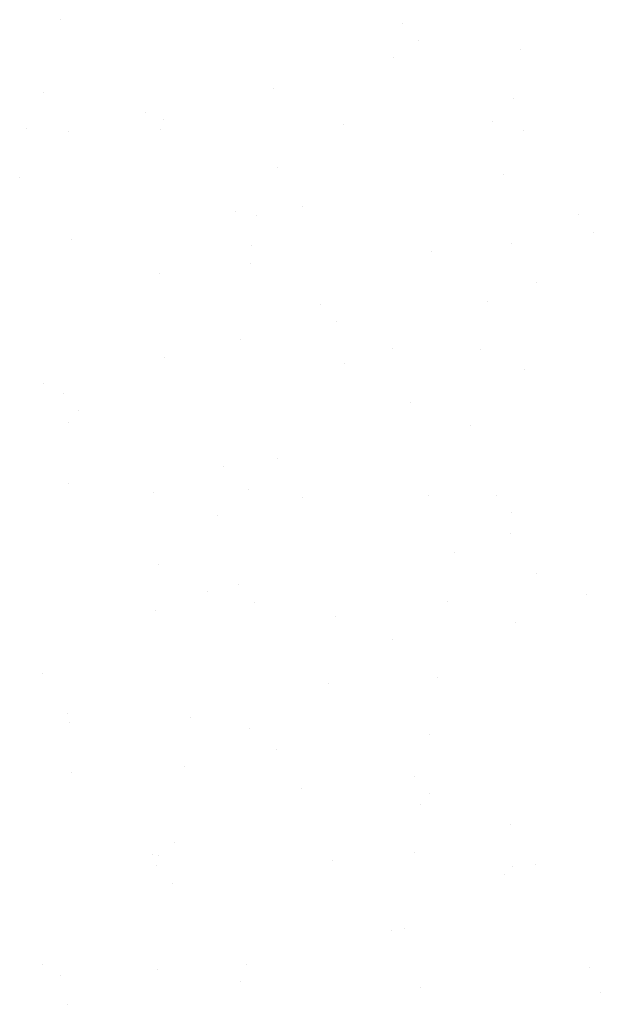
# Model space of a CAD drawing. Units: millimetres. Extents: x -857 to 54106, y -13666 to 13947.
# Tile 31 of 41: x 31340 to 31621, y 8976 to 9452. Entities that reach past the tile are written whole.
import ezdxf

# ---------------------------------------------------------------- set-up
doc = ezdxf.new("R2010")
doc.units = ezdxf.units.MM
doc.layers.add('A-FURN', color=21, linetype='Continuous', lineweight=18)
doc.layers.add('A-HT', color=15, linetype='Continuous')

# ---------------------------------------------------------------- blocks, each defined once
blk = doc.blocks.new('*X18')
at = {"color": 0}
for p, q in [((2.42041, 2.51943), (2.42041, 2.51943)), ((2.44643, 2.52286), (2.44643, 2.52286)), ((2.40072, 2.51004), (2.40072, 2.51004)), ((2.55643, 2.51033), (2.55643, 2.51033)), ((2.71213, 2.51061), (2.71213, 2.51061)), ((2.86784, 2.51089), (2.86784, 2.51089)), ((2.36196, 2.50128), (2.36196, 2.50128)), ((2.56203, 2.49956), (2.56203, 2.49956)), ((2.8734, 2.50111), (2.8734, 2.50111)), ((2.42181, 2.49661), (2.42181, 2.49661)), ((2.47957, 2.49519), (2.47957, 2.49519)), ((2.57751, 2.49689), (2.57751, 2.49689)), ((2.61045, 2.49686), (2.61045, 2.49686)), ((2.73322, 2.49718), (2.73322, 2.49718)), ((2.73835, 2.49625), (2.73835, 2.49625)), ((2.76505, 2.49514), (2.76505, 2.49514)), ((2.88893, 2.49746), (2.88893, 2.49746)), ((2.57125, 2.49112), (2.57125, 2.49112)), ((2.41172, 2.45568), (2.41172, 2.45568)), ((2.61474, 2.45126), (2.61474, 2.45126)), ((2.80894, 2.45165), (2.80894, 2.45165)), ((2.41511, 2.44573), (2.41511, 2.44573)), ((2.42094, 2.44723), (2.42094, 2.44723)), ((2.49771, 2.44825), (2.49771, 2.44825)), ((2.65342, 2.44854), (2.65342, 2.44854)), ((2.67806, 2.44998), (2.67806, 2.44998)), ((2.80912, 2.44882), (2.80912, 2.44882)), ((2.81482, 2.44954), (2.81482, 2.44954)), ((2.87027, 2.4492), (2.87027, 2.4492)), ((2.54301, 2.44511), (2.54301, 2.44511)), ((2.80236, 2.44026), (2.80236, 2.44026)), ((2.82403, 2.44109), (2.82403, 2.44109)), ((2.76171, 2.43491), (2.76171, 2.43491)), ((2.73568, 2.43148), (2.73568, 2.43148)), ((2.66777, 2.42254), (2.66777, 2.42254)), ((2.60109, 2.41376), (2.60109, 2.41376)), ((2.62712, 2.41719), (2.62712, 2.41719)), ((2.46444, 2.40737), (2.46444, 2.40737)), ((2.53318, 2.40482), (2.53318, 2.40482)), ((2.66451, 2.40565), (2.66451, 2.40565)), ((2.87655, 2.40477), (2.87655, 2.40477)), ((2.48272, 2.39885), (2.48272, 2.39885)), ((2.49253, 2.39947), (2.49253, 2.39947)), ((2.6136, 2.40052), (2.6136, 2.40052)), ((2.7415, 2.3999), (2.7415, 2.3999)), ((2.86753, 2.40123), (2.86753, 2.40123)), ((2.46651, 2.39604), (2.46651, 2.39604)), ((2.67373, 2.39721), (2.67373, 2.39721)), ((2.39859, 2.3871), (2.39859, 2.3871)), ((2.4411, 2.38484), (2.4411, 2.38484)), ((2.59681, 2.38512), (2.59681, 2.38512)), ((2.75252, 2.38541), (2.75252, 2.38541)), ((2.46219, 2.37141), (2.46219, 2.37141)), ((2.61789, 2.37169), (2.61789, 2.37169)), ((2.7736, 2.37197), (2.7736, 2.37197)), ((2.5142, 2.36177), (2.5142, 2.36177)), ((2.71723, 2.35735), (2.71723, 2.35735)), ((2.52342, 2.35332), (2.52342, 2.35332)), ((2.68121, 2.35364), (2.68121, 2.35364)), ((2.81209, 2.35531), (2.81209, 2.35531)), ((2.41826, 2.34939), (2.41826, 2.34939)), ((2.54616, 2.34877), (2.54616, 2.34877)), ((2.38238, 2.32277), (2.38238, 2.32277)), ((2.53809, 2.32305), (2.53809, 2.32305)), ((2.6938, 2.32333), (2.6938, 2.32333)), ((2.84951, 2.32362), (2.84951, 2.32362)), ((2.3639, 2.31789), (2.3639, 2.31789)), ((2.56692, 2.31347), (2.56692, 2.31347)), ((2.84846, 2.31687), (2.84846, 2.31687)), ((2.37311, 2.30944), (2.37311, 2.30944)), ((2.76699, 2.31175), (2.76699, 2.31175)), ((2.80781, 2.31152), (2.80781, 2.31152)), ((2.8797, 2.30843), (2.8797, 2.30843)), ((2.61675, 2.30418), (2.61675, 2.30418)), ((2.74465, 2.30356), (2.74465, 2.30356)), ((2.77621, 2.3033), (2.77621, 2.3033)), ((2.78178, 2.30809), (2.78178, 2.30809)), ((2.48587, 2.30251), (2.48587, 2.30251)), ((2.71387, 2.29915), (2.71387, 2.29915)), ((2.67322, 2.2938), (2.67322, 2.2938)), ((2.64719, 2.29037), (2.64719, 2.29037)), ((2.57928, 2.28143), (2.57928, 2.28143)), ((2.5126, 2.27265), (2.5126, 2.27265)), ((2.53863, 2.27608), (2.53863, 2.27608)), ((2.41661, 2.26958), (2.41661, 2.26958)), ((2.61669, 2.26786), (2.61669, 2.26786)), ((2.44469, 2.26371), (2.44469, 2.26371)), ((2.81971, 2.26344), (2.81971, 2.26344)), ((2.40404, 2.25836), (2.40404, 2.25836)), ((2.48148, 2.25963), (2.48148, 2.25963)), ((2.6259, 2.25942), (2.6259, 2.25942)), ((2.63719, 2.25992), (2.63719, 2.25992)), ((2.68436, 2.2573), (2.68436, 2.2573)), ((2.7929, 2.2602), (2.7929, 2.2602)), ((2.81524, 2.25897), (2.81524, 2.25897)), ((2.37802, 2.25493), (2.37802, 2.25493)), ((2.42141, 2.25304), (2.42141, 2.25304)), ((2.54931, 2.25243), (2.54931, 2.25243)), ((2.50257, 2.2462), (2.50257, 2.2462)), ((2.65828, 2.24648), (2.65828, 2.24648)), ((2.81398, 2.24677), (2.81398, 2.24677)), ((2.46638, 2.22398), (2.46638, 2.22398)), ((2.6694, 2.21956), (2.6694, 2.21956)), ((2.4756, 2.21553), (2.4756, 2.21553)), ((2.86947, 2.21784), (2.86947, 2.21784)), ((2.88285, 2.21209), (2.88285, 2.21209))]:
    blk.add_line(p, q, dxfattribs=at)
blk = doc.blocks.new('A$C6796526C')
at = {"layer": 'A-HT', "extrusion": (0, 0, -1), "zscale": -1, "rotation": 180}
blk.add_blockref('*X18', (0.55, 3), dxfattribs=at)

msp = doc.modelspace()

# ---------------------------------------------------------------- block references
at = {"layer": 'A-FURN', "xscale": 903.6084929786902, "yscale": 903.6084929786902, "zscale": 903.6084929786902, "rotation": 269.9999999999988}
msp.add_blockref('A$C6796526C', (30909.253, 11089.463), dxfattribs=at)

doc.saveas('drawing.dxf')
